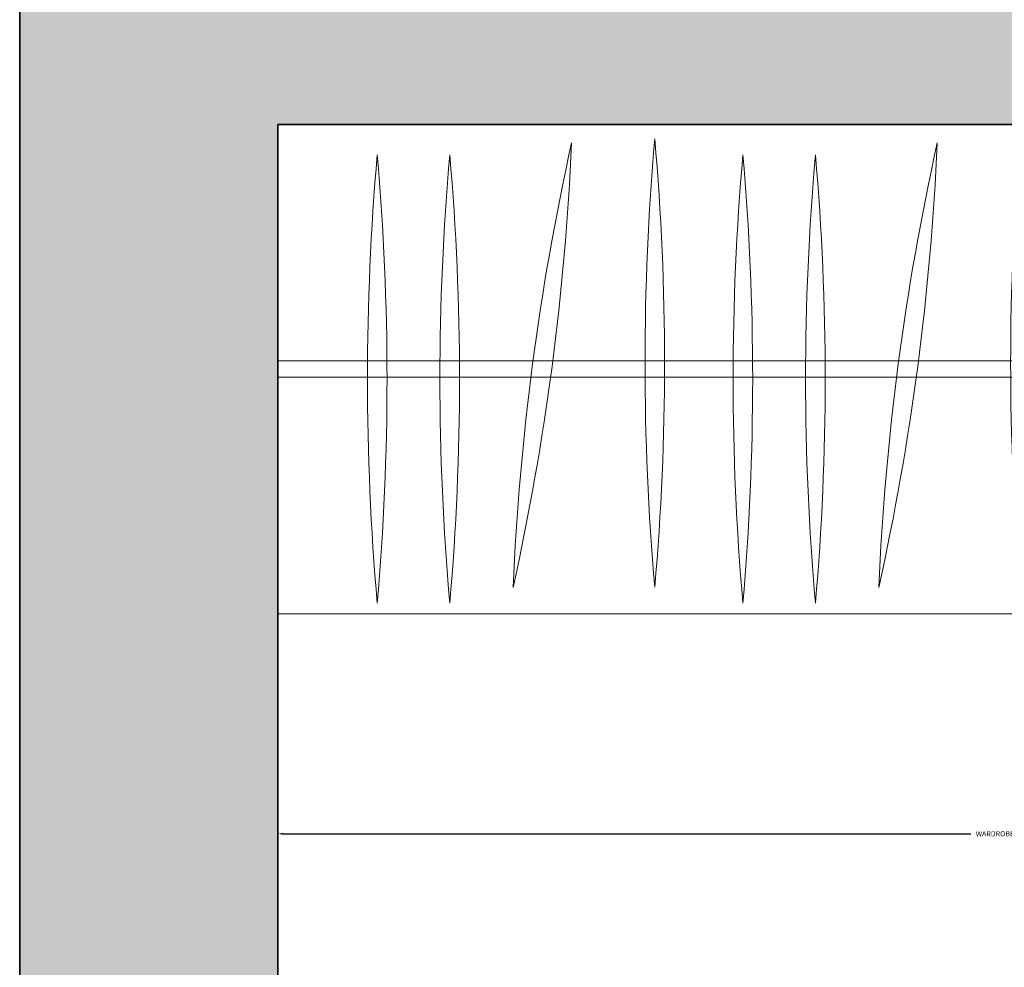
# Model space of a CAD drawing. Units: inches. Extents: x -9 to 505, y -680 to 48.
# Tile 9 of 17: x 27 to 62, y -198 to -165. Entities that reach past the tile are written whole.
import ezdxf

# ---------------------------------------------------------------- set-up
doc = ezdxf.new("R2010")
doc.units = ezdxf.units.IN
doc.header["$MEASUREMENT"] = 0
for name, color, linetype, lineweight in [('A-ANNO-DIMS', 2, 'Continuous', 18), ('A-FLOR-CASE', 8, 'Continuous', 18), ('A-WALL', 7, 'Continuous', 35), ('A-WALL-PATT', 251, 'Continuous', 13)]:
    doc.layers.add(name, color=color, linetype=linetype, lineweight=lineweight)
doc.styles.get("Standard").update_dxf_attribs({"font": 'arial.ttf'})
doc.dimstyles.get("Standard").update_dxf_attribs({"dimtxt": 0.18, "dimasz": 0.18, "dimexe": 0.18, "dimexo": 0.0625, "dimgap": 0.09, "dimtad": 0, "dimtih": 1, "dimtoh": 1, "dimdec": 0, "dimzin": 0, "dimdsep": 46, "dimlunit": 3, "dimtxsty": 'Standard', "dimcen": 0.09, "dimadec": 0, "dimazin": 0, "dimtfac": 1, "dimtdec": 0, "dimtofl": 0, "dimtmove": 0, "dimatfit": 3, "dimfxl": 1, "dimtolj": 1, "dimtzin": 0, "dimarcsym": 0})

# ---------------------------------------------------------------- blocks, each defined once
blk = doc.blocks.new('*D3')
at = {"layer": 'A-ANNO-DIMS', "color": 0, "lineweight": -2, "transparency": 16777216}
for p, q in [((27.201, 11.499), (5.161, 11.499)), ((5.341, 11.319), (5.341, -330.86)), ((5.341, -679.321), (5.341, -337.142)), ((27.201, -679.501), (5.161, -679.501))]:
    blk.add_line(p, q, dxfattribs=at)
at = {"layer": 'A-ANNO-DIMS', "color": 0, "transparency": 16777216}
for points in [[(5.311, 11.319), (5.371, 11.319), (5.341, 11.499)], [(5.311, -679.321), (5.371, -679.321), (5.341, -679.501)]]:
    blk.add_solid(points, dxfattribs=at)
at = {"layer": 'Defpoints', "color": 0, "transparency": 16777216}
for p in [(27.264, 11.499), (5.341, -679.501), (27.264, -679.501)]:
    blk.add_point(p, dxfattribs=at)
at = {"layer": 'A-ANNO-DIMS', "color": 0, "transparency": 16777216, "insert": (5.341, -334.001), "char_height": 6, "attachment_point": 5}
blk.add_mtext('\\A1;57\'-7"', dxfattribs=at)
blk = doc.blocks.new('WARDROBE-HANGING')
for p, q in [((51.194, 17.065), (0, 17.065)), ((0, 17.065), (0, 0)), ((51.194, 17.065), (51.194, 0)), ((51.194, 8.817), (0, 8.817)), ((51.194, 8.248), (0, 8.248)), ((51.194, 0), (0, 0))]:
    blk.add_line(p, q)
for centre, start, end in [((102.603, 8.742), 175.00281, 184.99719), ((-76.297, 8.742), 355.00281, 4.99719), ((115.358, 8.742), 175.00281, 184.99719), ((-63.542, 8.742), 355.00281, 4.99719), ((128.16, 8.742), 175.00281, 184.99719), ((-50.739, 8.742), 355.00281, 4.99719), ((-79.455, 20.34), 347.50795, 357.50233), ((97.917, -2.996), 167.50795, 177.50233), ((-66.699, 20.34), 347.50795, 357.50233), ((110.672, -2.996), 167.50795, 177.50233), ((123.474, -2.996), 167.50795, 177.50233), ((-53.897, 20.34), 347.50795, 357.50233), ((136.229, -2.996), 167.50795, 177.50233), ((-41.142, 20.34), 347.50795, 357.50233), ((92.922, 8.192), 175.00281, 184.99719), ((-85.978, 8.192), 355.00281, 4.99719), ((95.45, 8.192), 175.00281, 184.99719), ((-83.449, 8.192), 355.00281, 4.99719), ((105.677, 8.192), 175.00281, 184.99719), ((-73.223, 8.192), 355.00281, 4.99719), ((108.205, 8.192), 175.00281, 184.99719), ((-70.694, 8.192), 355.00281, 4.99719), ((118.479, 8.192), 175.00281, 184.99719), ((-60.421, 8.192), 355.00281, 4.99719), ((121.008, 8.192), 175.00281, 184.99719), ((-57.892, 8.192), 355.00281, 4.99719), ((131.234, 8.192), 175.00281, 184.99719), ((-47.666, 8.192), 355.00281, 4.99719), ((133.763, 8.192), 175.00281, 184.99719), ((-45.137, 8.192), 355.00281, 4.99719)]:
    blk.add_arc(centre, 89.791, start, end)
blk = doc.blocks.new('*D22')
at = {"layer": 'A-ANNO-DIMS', "color": 0, "lineweight": -2, "transparency": 16777216}
for p, q in [((36.264, -185.628), (36.264, -193.425)), ((87.458, -185.628), (87.458, -193.425)), ((36.444, -193.245), (60.443, -193.245)), ((87.278, -193.245), (63.279, -193.245))]:
    blk.add_line(p, q, dxfattribs=at)
at = {"layer": 'A-ANNO-DIMS', "color": 0, "transparency": 16777216}
for points in [[(36.444, -193.215), (36.444, -193.275), (36.264, -193.245)], [(87.278, -193.215), (87.278, -193.275), (87.458, -193.245)]]:
    blk.add_solid(points, dxfattribs=at)
at = {"layer": 'Defpoints', "color": 0, "transparency": 16777216}
for p in [(36.264, -185.566), (87.458, -185.566), (87.458, -193.245)]:
    blk.add_point(p, dxfattribs=at)
at = {"layer": 'A-ANNO-DIMS', "color": 0, "transparency": 16777216, "insert": (61.861, -193.245), "char_height": 0.18, "attachment_point": 5}
blk.add_mtext('\\A1;WARDROBE 4\'-3" TYP.', dxfattribs=at)

msp = doc.modelspace()

# ---------------------------------------------------------------- hatches: boundary and pattern name
at = {"layer": 'A-WALL-PATT'}
h = msp.add_hatch(color=256, dxfattribs=at)
h.dxf.hatch_style = 1
h.paths.add_polyline_path([(101.641, 11.499), (48.264, 11.499), (48.264, 2.499), (72.264, 2.499), (72.264, -21.248), (81.264, -21.248), (81.264, 2.499), (101.641, 2.499)])
h.paths.add_polyline_path([(36.264, 2.499), (27.264, 2.499), (27.264, -6.918), (36.264, -6.918)])
h.paths.add_polyline_path([(81.264, -57.248), (72.264, -57.248), (72.264, -75.501), (81.264, -75.501)])
h.paths.add_polyline_path([(162.764, 11.499), (137.641, 11.499), (137.641, 2.499), (162.764, 2.499)])
h.paths.add_polyline_path([(179.264, 2.499), (174.764, 2.499), (174.764, -75.501), (179.264, -75.501), (179.264, -54.501), (229.514, -54.501), (229.514, -45.501), (179.264, -45.501)])
h.paths.add_polyline_path([(382.256, -45.501), (332.264, -45.501), (332.264, 2.499), (327.764, 2.499), (327.764, -45.501), (277.514, -45.501), (277.514, -54.501), (327.764, -54.501), (327.764, -111.501), (332.264, -111.501), (332.264, -54.501), (382.256, -54.501)])
h.paths.add_polyline_path([(332.264, -128.001), (327.764, -128.001), (327.764, -207.001), (332.264, -207.001)])
h.paths.add_polyline_path([(124.764, -111.501), (36.264, -111.501), (36.264, -116.001), (120.264, -116.001), (120.264, -168.501), (179.264, -168.501), (179.264, -164.001), (124.764, -164.001)])
h.paths.add_polyline_path([(96.264, -164.001), (36.264, -164.001), (36.264, -152.001), (27.264, -152.001), (27.264, -208.879), (36.264, -208.879), (36.264, -168.501), (96.264, -168.501)])
h.paths.add_polyline_path([(36.264, -244.879), (27.264, -244.879), (27.264, -287.001), (36.264, -287.001)])
h.paths.add_polyline_path([(179.264, -204.501), (174.764, -204.501), (174.764, -287.001), (179.264, -287.001)])
h.paths.add_polyline_path([(257.264, -296.001), (248.264, -296.001), (248.264, -446.001), (269.264, -446.001), (269.264, -437.001), (257.264, -437.001)])
h.paths.add_polyline_path([(90.264, -296.001), (81.264, -296.001), (81.264, -348.67), (90.264, -348.67)])
h.paths.add_polyline_path([(90.264, -384.67), (81.264, -384.67), (81.264, -416.001), (90.264, -416.001)])
h.paths.add_polyline_path([(170.264, -452.001), (36.264, -452.001), (36.264, -456.501), (165.764, -456.501), (165.764, -504.501), (165.133, -504.501), (165.133, -509.001), (170.264, -509.001)])
h.paths.add_polyline_path([(141.764, -504.501), (36.264, -504.501), (36.264, -492.501), (27.264, -492.501), (27.264, -565.959), (36.264, -565.959), (36.264, -509.001), (141.764, -509.001)])
h.paths.add_polyline_path([(36.264, -601.959), (27.264, -601.959), (27.264, -658.501), (36.264, -658.501)])
h.paths.add_polyline_path([(170.264, -670.501), (170.264, -634.501), (222.764, -634.501), (222.764, -625.501), (165.764, -625.501), (165.764, -670.501), (36.264, -670.501), (36.264, -679.501), (170.264, -679.501)])
h.paths.add_polyline_path([(332.264, -616.501), (433.894, -616.501), (433.894, -612.001), (332.264, -612.001), (332.264, -610.563), (327.764, -610.563), (327.764, -625.501), (270.764, -625.501), (270.764, -634.501), (327.764, -634.501), (327.764, -658.501), (332.264, -658.501)])
h.paths.add_polyline_path([(459.764, -670.501), (336.764, -670.501), (336.764, -679.501), (459.764, -679.501)])
h.paths.add_polyline_path([(468.764, -545.737), (459.764, -545.737), (459.764, -612.001), (457.894, -612.001), (457.894, -616.501), (459.764, -616.501), (459.764, -658.501), (468.764, -658.501)])
h.paths.add_polyline_path([(332.264, -446.001), (327.764, -446.001), (327.764, -574.563), (332.264, -574.563)])
h.paths.add_polyline_path([(327.764, -437.001), (305.264, -437.001), (305.264, -446.001), (327.764, -446.001)])
h.paths.add_polyline_path([(459.764, -437.001), (348.764, -437.001), (348.764, -446.001), (459.764, -446.001)])
h.paths.add_polyline_path([(468.764, -458.001), (459.764, -458.001), (459.764, -509.737), (468.764, -509.737)])
h.paths.add_polyline_path([(468.764, -365.001), (459.764, -365.001), (459.764, -437.001), (468.764, -437.001)])
h.paths.add_polyline_path([(468.764, -299.601), (459.764, -299.601), (459.764, -344.001), (468.764, -344.001)])
h.paths.add_polyline_path([(468.764, -184.739), (459.764, -184.739), (459.764, -231.001), (401.264, -231.001), (401.264, -235.501), (459.764, -235.501), (459.764, -275.601), (468.764, -275.601)])
h.paths.add_polyline_path([(390.764, -356.001), (342.764, -356.001), (342.764, -365.001), (390.764, -365.001)])
h.paths.add_polyline_path([(459.764, -356.001), (405.764, -356.001), (405.764, -365.001), (459.764, -365.001)])
h.paths.add_polyline_path([(405.764, -296.001), (396.764, -296.001), (396.764, -356.001), (405.764, -356.001)])
h.paths.add_polyline_path([(336.764, -296.001), (327.764, -296.001), (327.764, -356.001), (336.764, -356.001)])
h.paths.add_polyline_path([(468.764, -9.501), (459.764, -9.501), (459.764, -45.501), (418.256, -45.501), (418.256, -54.501), (468.764, -54.501)])
h.paths.add_polyline_path([(468.764, -54.501), (459.764, -54.501), (459.764, -111.501), (468.764, -111.501)])
h.paths.add_polyline_path([(468.764, -128.001), (459.764, -128.001), (459.764, -148.739), (468.764, -148.739)])

# ---------------------------------------------------------------- linework, layer by layer
at = {"layer": 'A-WALL'}
for p, q in [((27.264, 11.499), (27.264, -679.501)), ((36.264, -168.501), (179.264, -168.501)), ((36.264, -168.501), (36.264, -287.001))]:
    msp.add_line(p, q, dxfattribs=at)

# ---------------------------------------------------------------- block references
at = {"layer": 'A-FLOR-CASE'}
msp.add_blockref('WARDROBE-HANGING', (36.264, -185.566), dxfattribs=at)

# ---------------------------------------------------------------- dimensions: what is measured, and where the dimension line sits
at = {"layer": 'A-ANNO-DIMS'}
dim = msp.add_linear_dim(base=(5.341, -679.501), p1=(27.264, 11.499), p2=(27.264, -679.501), angle=90, dimstyle='Standard', override={"dimtxt": 6, "dimclrd": 0, "dimclre": 0, "dimclrt": 0}, dxfattribs=at)
dim.commit()
dim.dimension.update_dxf_attribs({"geometry": '*D3', "text_midpoint": (5.341, -334.001)})
dim = msp.add_linear_dim(base=(87.458, -193.245), p1=(36.264, -185.566), p2=(87.458, -185.566), text='WARDROBE <> TYP.', dimstyle='Standard', override={"dimdec": 1, "dimlfac": 1, "dimrnd": 0, "dimzin": 1, "dimdsep": 46, "dimlunit": 4, "dimfrac": 2}, dxfattribs=at)
dim.commit()
dim.dimension.update_dxf_attribs({"geometry": '*D22', "text_midpoint": (61.861, -193.245)})

doc.saveas('drawing.dxf')
